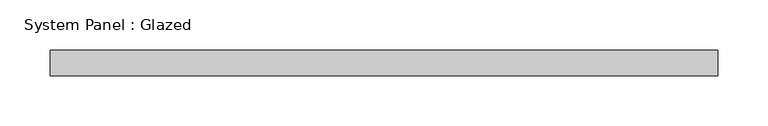
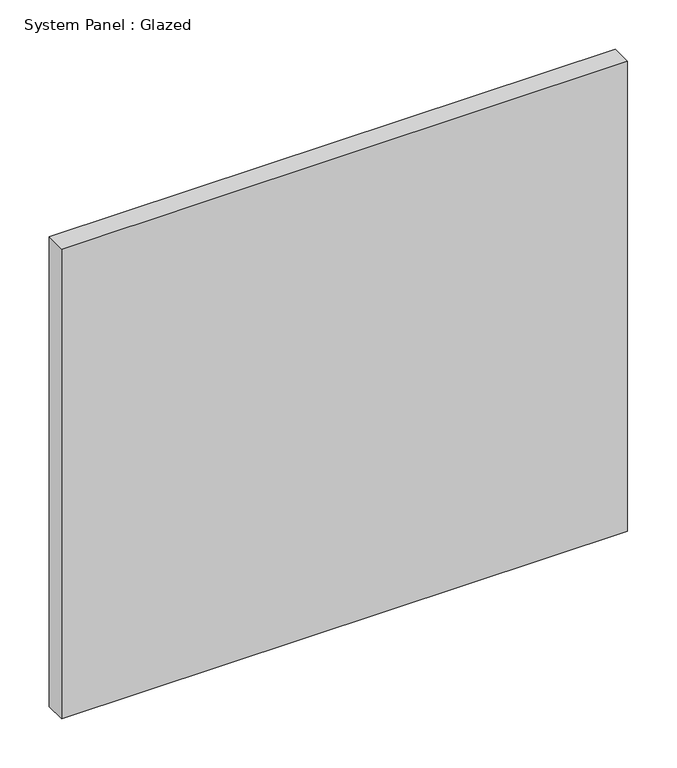
"""IFC4 building model written with IfcOpenShell, lengths in millimetres: plate geometry, System Panel : Glazed."""

from ifc_helpers import new_model, si_unit, origin, origin_with_axes, place, context, project, spatial, polyline, outline, extrude, source, transform, mapped, element, save


def system_panel_glazed_4819e94b(model_context):
    return source(origin(), model_context, "Body", "SweptSolid", [
        extrude(outline(polyline([(333.375, 19.05), (-333.375, 19.05), (-333.375, 44.45), (333.375, 44.45), (333.375, 19.05)])), origin_with_axes(), (0.0, 0.0, 1.0), 584.7888769),
    ])


if __name__ == "__main__":
    model = new_model("IFC4")
    model_context = context("Model", 3, world=origin())
    ifc_project = project(units=[si_unit("LENGTHUNIT", "METRE", prefix="MILLI")], contexts=[model_context])
    site = spatial("IfcSite", under=ifc_project)
    building = spatial("IfcBuilding", under=site)
    placement = place(None, origin())
    system_panel_glazed_shape = system_panel_glazed_4819e94b(model_context)
    element("IfcPlate", 1, ObjectType="System Panel : Glazed", at=placement, inside=building, context=model_context, shape_type="MappedRepresentation", body=[
        mapped(system_panel_glazed_shape, transform((0.0, 0.0, 0.0), x_axis=(1.0, 0.0, 0.0), y_axis=(0.0, 1.0, 0.0), z_axis=(0.0, 0.0, 1.0))),
    ])
    save(model, "model.ifc")

# Revit data of these elements
# Type "System Panel : Glazed"
#   Construction Type Id = "GSP4R"
#   Analytic Construction = "1/8 in Pilkington single glazing"
#   Visual Light Transmittance = 0.9
#   Solar Heat Gain Coefficient = 0.86
#   Heat Transfer Coefficient (U) = 1.18115 BTU/(h·ft²·°F)
#   Define Thermal Properties by = 1
# Element 1 (IfcPlate, "System Panel : Glazed")
#   Materials on its faces: "Glass"
# Materials
#   "Glass": class "Glass", colour RGB 0 128 192, transparency 0.75, Description = "Soda Lime Glass", Cost = 0
